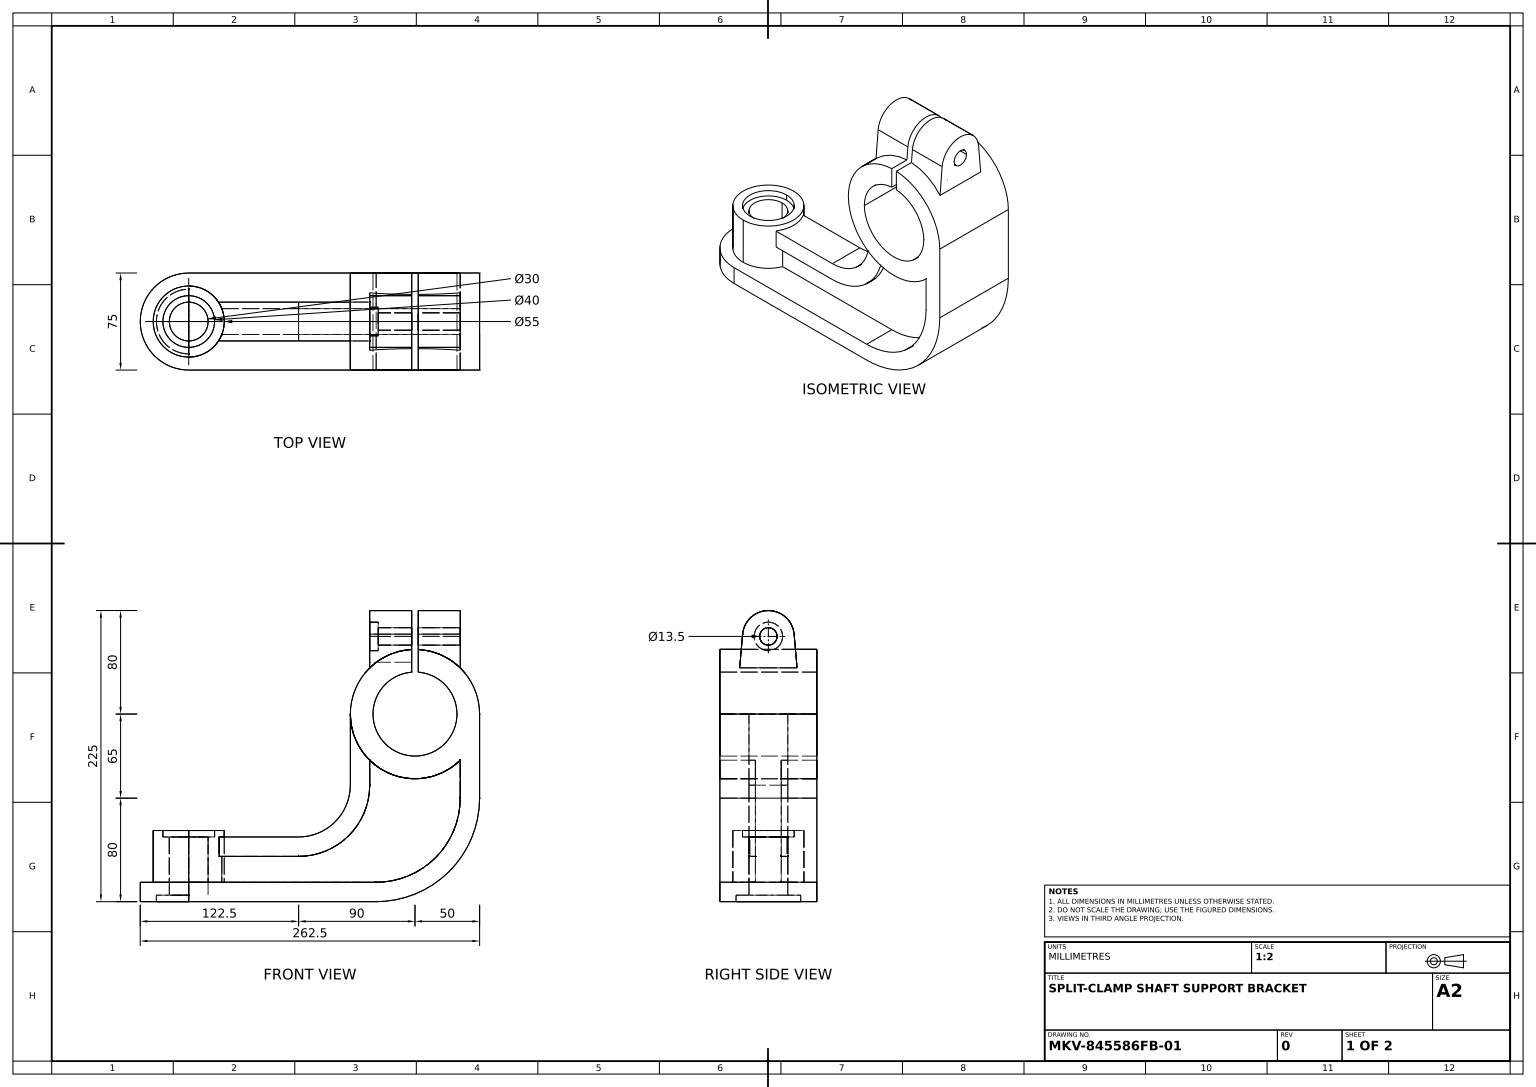
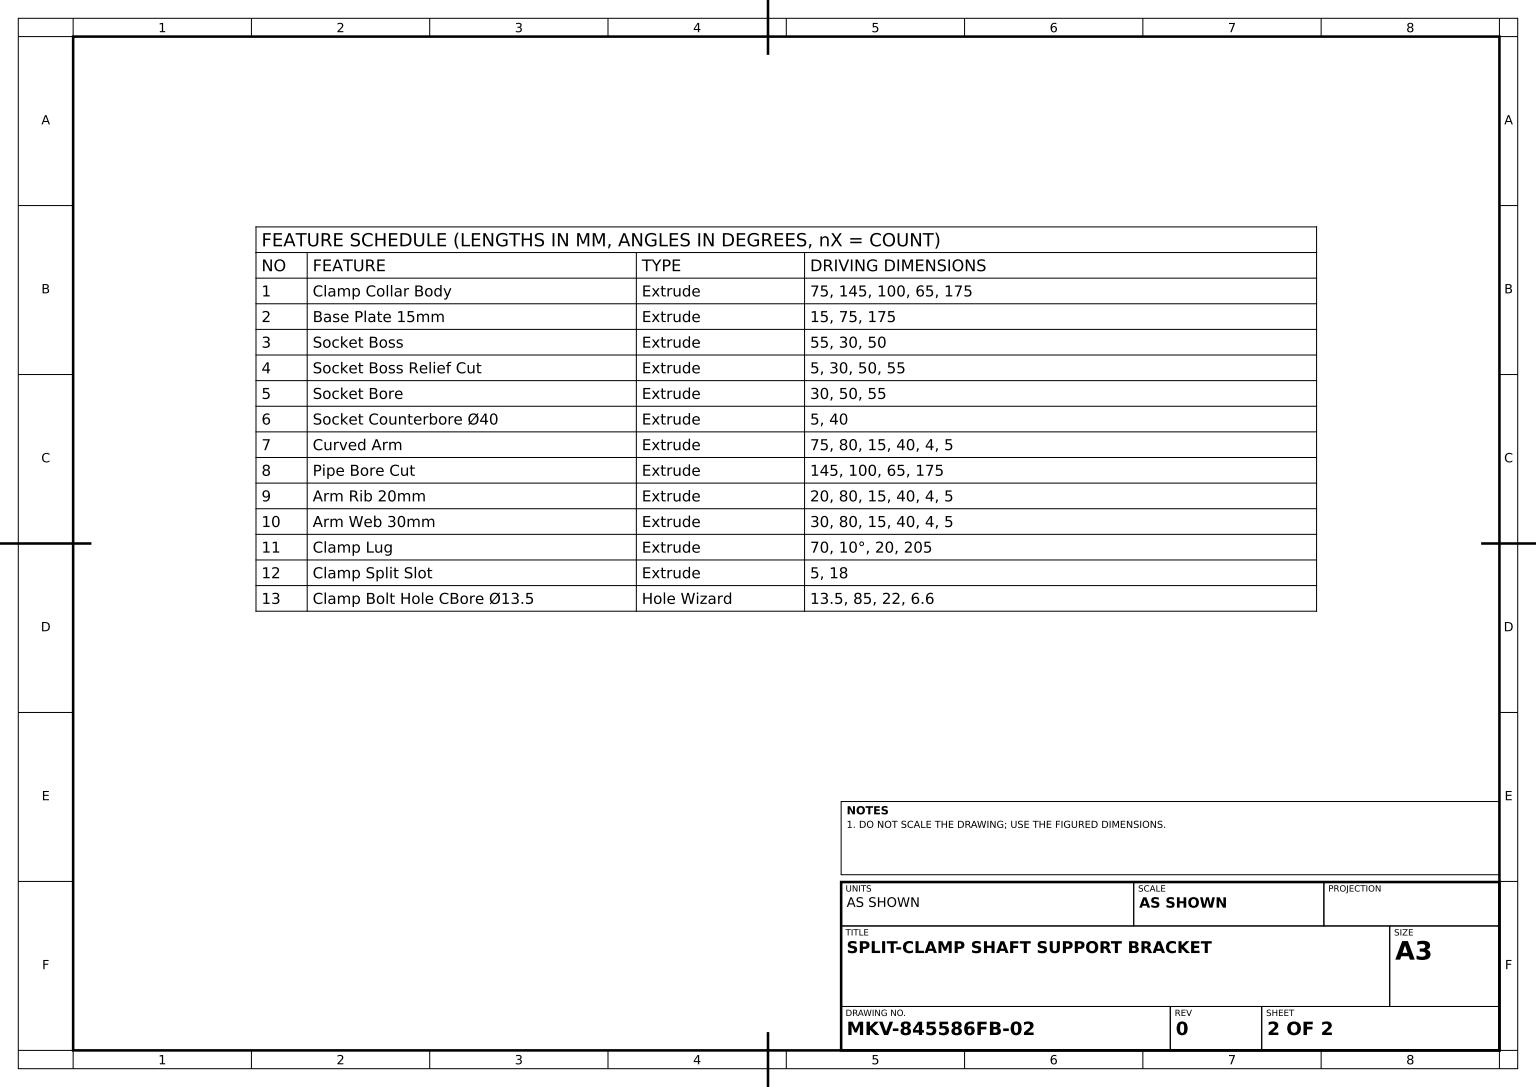
from build123d import *

# Parameters (mm, degrees)
MOUNT_SIDE_PROFILE_SKETCH_R            = 50
MOUNT_SIDE_PROFILE_SKETCH_R_2          = 32.5
CLAMP_COLLAR_BODY_DEPTH                = 37.5
BASE_PLATE_SKETCH_R                    = 37.5
BASE_PLATE_15MM_DEPTH                  = 15
SOCKET_BOSS_SKETCH_R                   = 27.5
SOCKET_BOSS_DEPTH                      = 55
SKETCH10_3_R                           = 25
SOCKET_BOSS_RELIEF_CUT_DEPTH           = 5
SOCKET_START                           = -55
SKETCH10_4_R                           = 15
SOCKET_BORE_DEPTH                      = 50
SOCKET_COUNTERBORE_SKETCH_40_R         = 20
SOCKET_COUNTERBORE_40_DEPTH            = 5
CURVED_ARM_DEPTH                       = 37.5
PIPE_BORE_CUT_DEPTH                    = 291.839302709
PIPE_BORE_CUT_DEPTH_BACK               = 291.839302709
SKETCH1_2_R                            = 32.5
ARM_RIB_20MM_DEPTH                     = 10
ARM_WEB_30MM_DEPTH                     = 15
CLAMP_LUG_DEPTH                        = 35
CLAMP_SPLIT_SLOT_DEPTH                 = 2.5
CLAMP_BOLT_HOLE_CBORE_13_5_D           = 13.5
CLAMP_BOLT_HOLE_CBORE_13_5_CBORE_D     = 22
CLAMP_BOLT_HOLE_CBORE_13_5_CBORE_DEPTH = 6.6


with BuildPart() as part:
    # Mount Side Profile Sketch → Clamp Collar Body (new, symmetric)
    with BuildSketch(Plane.XY):
        with Locations((0, 145)):
            Circle(MOUNT_SIDE_PROFILE_SKETCH_R)
        with Locations((0, 145)):
            Circle(MOUNT_SIDE_PROFILE_SKETCH_R_2, mode=Mode.SUBTRACT)
    extrude(amount=CLAMP_COLLAR_BODY_DEPTH, both=True)



with BuildPart() as body_2:
    # Base Plate Sketch → Base Plate 15mm (new body)
    with BuildSketch(Plane(origin=(0, 0, 0), x_dir=(1, 0, 0), z_dir=(0, 1, 0))):
        with Locations(Location((-175, 0, 0), (0, 0, 270))):
            Circle(BASE_PLATE_SKETCH_R)
    extrude(amount=BASE_PLATE_15MM_DEPTH)

    # Socket Boss Sketch → Socket Boss (add)
    with BuildSketch(Plane.XZ):
        with Locations(Location((-175, 0, 0), (0, 0, 270))):
            Circle(SOCKET_BOSS_SKETCH_R)
    extrude(amount=-SOCKET_BOSS_DEPTH)

    # Sketch10_3 → Socket Boss Relief Cut (cut)
    with BuildSketch(Plane.XZ):
        with Locations(Location((-175, 0, 0), (0, 0, 270))):
            Circle(SKETCH10_3_R)
    extrude(amount=-SOCKET_BOSS_RELIEF_CUT_DEPTH, mode=Mode.SUBTRACT)

    # Sketch10_4 → Socket Bore (cut)
    with BuildSketch(Plane.XZ.offset(SOCKET_START)):
        with Locations(Location((-175, 0, 0), (0, 0, 270))):
            Circle(SKETCH10_4_R)
    extrude(amount=SOCKET_BORE_DEPTH, mode=Mode.SUBTRACT)

    # Socket Counterbore Sketch _40 → Socket Counterbore _40 (cut)
    with BuildSketch(Plane(origin=(0, 55, 0), x_dir=(1, 0, 0), z_dir=(0, 1, 0))):
        with Locations(Location((-175, 0, 0), (0, 0, 270))):
            Circle(SOCKET_COUNTERBORE_SKETCH_40_R)
    extrude(amount=-SOCKET_COUNTERBORE_40_DEPTH, mode=Mode.SUBTRACT)


with BuildPart() as part_1:
    add(part.part)

    add(body_2.part)  # Curved Arm merges body 2
    # Curved Arm Profile Sketch → Curved Arm (add, symmetric)
    with BuildSketch(Plane.XY):
        with BuildLine():
            Line((-175, 0), (-30, 0))
            ThreePointArc((-30, 0), (26.568542495, 23.431457505), (50, 80))
            Line((50, 80), (50, 145))
            ThreePointArc((50, 145), (-46.097722286, 164.364916731), (35, 109.292857857))
            Line((35, 109.292857857), (35, 80))
            ThreePointArc((35, 80), (15.961940777, 34.038059223), (-30, 15))
            Line((-30, 15), (-175, 15))
            Line((-175, 15), (-175, 0))
        make_face()
    extrude(amount=CURVED_ARM_DEPTH, both=True)

    # Sketch1_2 → Pipe Bore Cut (cut, two sides: drawn at the far end of the back side and taken through both)
    with BuildSketch(Plane.XY.offset(-PIPE_BORE_CUT_DEPTH_BACK)):
        with Locations((0, 145)):
            Circle(SKETCH1_2_R)
    extrude(amount=PIPE_BORE_CUT_DEPTH + PIPE_BORE_CUT_DEPTH_BACK, mode=Mode.SUBTRACT)

    # Sketch12_3 → Arm Rib 20mm (add, symmetric)
    with BuildSketch(Plane.XY):
        with BuildLine():
            Line((-151.5, 35), (-151.5, 15))
            Line((-151.5, 15), (-30, 15))
            ThreePointArc((-30, 15), (15.961940777, 34.038059223), (35, 80))
            Line((35, 80), (35, 109.292857857))
            ThreePointArc((35, 109.292857857), (0, 95), (-35, 109.292857857))
            Line((-35, 109.292857857), (-35, 90))
            ThreePointArc((-35, 90), (-51.109127035, 51.109127035), (-90, 35))
            Line((-90, 35), (-151.5, 35))
        make_face()
    extrude(amount=ARM_RIB_20MM_DEPTH, both=True)

    # Sketch12_4 → Arm Web 30mm (add, symmetric)
    with BuildSketch(Plane.XY):
        with BuildLine():
            Line((-151.5, 50), (-151.5, 35))
            Line((-151.5, 35), (-90, 35))
            ThreePointArc((-90, 35), (-51.109127035, 51.109127035), (-35, 90))
            Line((-35, 90), (-35, 109.292857857))
            ThreePointArc((-35, 109.292857857), (-46.097722286, 125.635083269), (-50, 145))
            Line((-50, 145), (-50, 90))
            ThreePointArc((-50, 90), (-61.715728753, 61.715728753), (-90, 50))
            Line((-90, 50), (-151.5, 50))
        make_face()
    extrude(amount=ARM_WEB_30MM_DEPTH, both=True)

    # Clamp Lug Sketch → Clamp Lug (add, symmetric)
    with BuildSketch(Plane(origin=(0, 0, 0), x_dir=(0, 0, -1), z_dir=(1, 0, 0))):
        with BuildLine():
            Line((19.923893962, 206.743114855), (22.482334998, 177.5))
            Line((22.482334998, 177.5), (-22.482334998, 177.5))
            Line((-22.482334998, 177.5), (-19.923893962, 206.743114855))
            ThreePointArc((-19.923893962, 206.743114855), (0, 225), (19.923893962, 206.743114855))
        make_face()
    extrude(amount=CLAMP_LUG_DEPTH, both=True)

    # Clamp Split Slot Sketch → Clamp Split Slot (cut, symmetric)
    with BuildSketch(Plane(origin=(0, 0, 0), x_dir=(0, 0, -1), z_dir=(1, 0, 0))):
        with BuildLine():
            Line((-37.855398527, 208.311918224), (-41.845299437, 162.707142143))
            Line((-41.845299437, 162.707142143), (41.845299437, 162.707142143))
            Line((41.845299437, 162.707142143), (37.855398527, 208.311918224))
            ThreePointArc((37.855398527, 208.311918224), (0, 243), (-37.855398527, 208.311918224))
        make_face()
    extrude(amount=CLAMP_SPLIT_SLOT_DEPTH, both=True, mode=Mode.SUBTRACT)

    # Clamp Bolt Hole CBore _13.5 (through all)
    with Locations(Plane.ZY.offset(35)):
        with Locations((0, 205)):
            CounterBoreHole(CLAMP_BOLT_HOLE_CBORE_13_5_D / 2, CLAMP_BOLT_HOLE_CBORE_13_5_CBORE_D / 2, CLAMP_BOLT_HOLE_CBORE_13_5_CBORE_DEPTH)


solid = part_1.part
